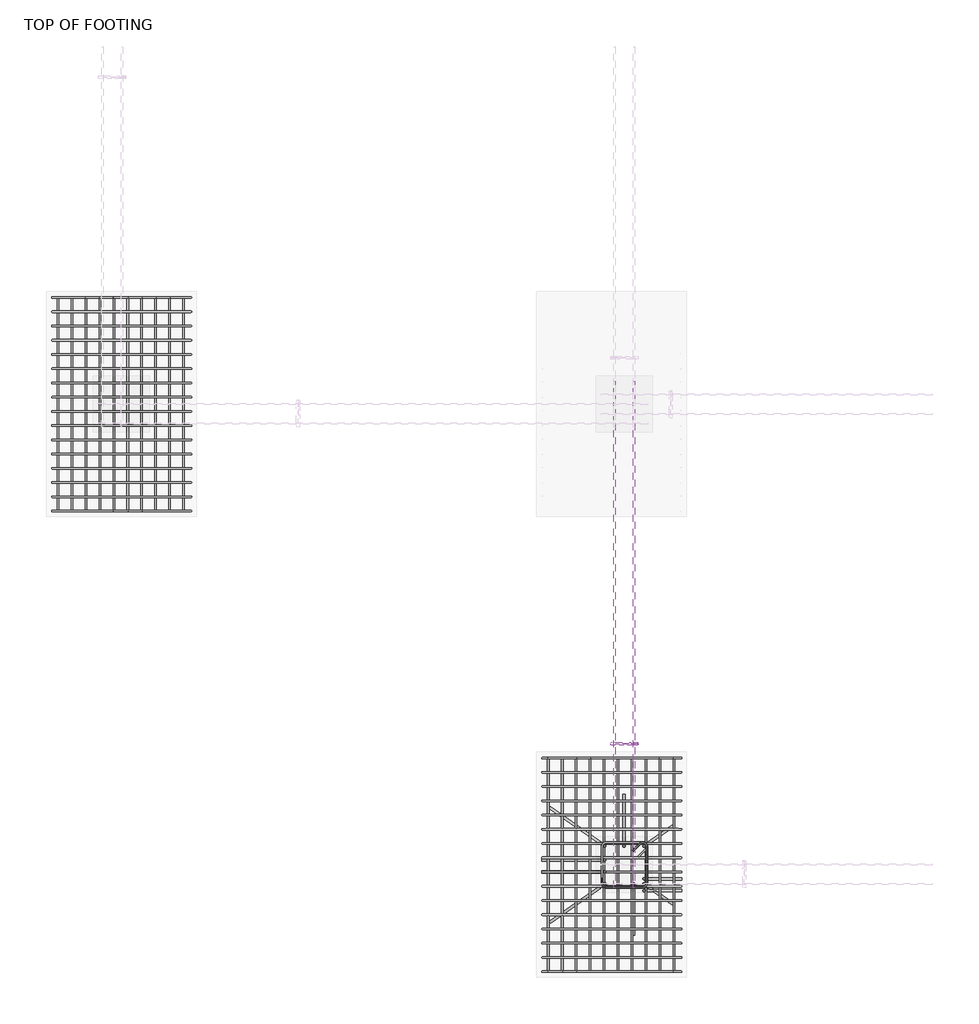
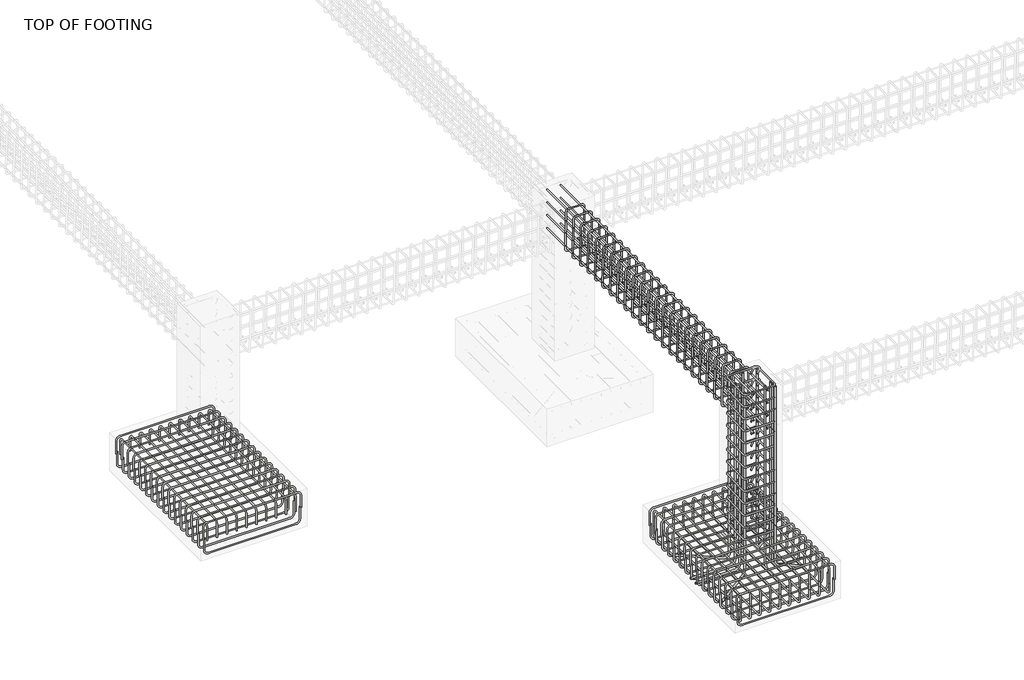
# One storey, part 2 of 11: 19 reinforcing bars.
"""IFC4 building model written with IfcOpenShell, lengths in millimetres."""

from ifc_helpers import new_model, si_unit, point, frame, origin, place, context, project, spatial, polyline, circle_curve, trimmed, segment, composite_curve, source, transform, mapped, element, save
from ifc_brep_helpers import swept_disk

model = new_model("IFC4")

# Units and contexts
model_context = context("Model", 3, world=origin())
ifc_project = project(units=[si_unit("LENGTHUNIT", "METRE", prefix="MILLI")], contexts=[model_context])

# Site, building, storey
site = spatial("IfcSite", under=ifc_project)
building = spatial("IfcBuilding", under=site)
storey = spatial("IfcBuildingStorey", under=building, Name="TOP OF FOOTING", Elevation=-1828.8)

# Reinforcing bars
placement = place(None, origin())
reinforcing_bar_shape = source(origin(), model_context, "Body", "SolidModel", [
    swept_disk(composite_curve([segment(polyline([(-5733.2210247, -2335.4013044, -2046.7466921), (-5733.2210247, -2335.4013044, -2194.0466921)]), True, "CONTINUOUS"), segment(trimmed(circle_curve(frame((-5779.5710247, -2335.4013044, -2194.0466921), z_axis=(0.0, 1.0, 0.0), x_axis=(46.349999999999454, 0.0, 0.0)), 46.35), [point((-5733.2210247, -2335.4013044, -2194.0466921))], [point((-5779.5710247, -2335.4013044, -2240.3966921))], True, "CARTESIAN"), True, "CONTINUOUS"), segment(polyline([(-5779.5710247, -2335.4013044, -2240.3966921), (-6770.7992774, -2335.4013044, -2240.3966921)]), True, "CONTINUOUS"), segment(trimmed(circle_curve(frame((-6770.7992774, -2335.4013044, -2194.0466921), z_axis=(0.0, 1.0, 0.0), x_axis=(0.0, 0.0, -46.34999999999991)), 46.35), [point((-6770.7992774, -2335.4013044, -2240.3966921))], [point((-6817.1492774, -2335.4013044, -2194.0466921))], True, "CARTESIAN"), True, "CONTINUOUS"), segment(polyline([(-6817.1492774, -2335.4013044, -2194.0466921), (-6817.1492774, -2335.4013044, -2046.7466921)]), True, "CONTINUOUS")], self_intersect=False), 6.35),
])
element("IfcReinforcingBar", 1, at=placement, inside=storey, context=model_context, shape_type="MappedRepresentation", body=[
    mapped(reinforcing_bar_shape, transform((0.0, 0.0, 0.0), x_axis=(1.0, 0.0, 0.0), y_axis=(0.0, 1.0, 0.0), z_axis=(0.0, 0.0, 1.0))),
    mapped(reinforcing_bar_shape, transform((0.0, -113.82, 0.0), x_axis=(1.0, 0.0, 0.0), y_axis=(0.0, 1.0, 0.0), z_axis=(0.0, 0.0, 1.0))),
    mapped(reinforcing_bar_shape, transform((0.0, -227.64, 0.0), x_axis=(1.0, 0.0, 0.0), y_axis=(0.0, 1.0, 0.0), z_axis=(0.0, 0.0, 1.0))),
    mapped(reinforcing_bar_shape, transform((0.0, -341.46, 0.0), x_axis=(1.0, 0.0, 0.0), y_axis=(0.0, 1.0, 0.0), z_axis=(0.0, 0.0, 1.0))),
    mapped(reinforcing_bar_shape, transform((0.0, -455.28, 0.0), x_axis=(1.0, 0.0, 0.0), y_axis=(0.0, 1.0, 0.0), z_axis=(0.0, 0.0, 1.0))),
    mapped(reinforcing_bar_shape, transform((0.0, -569.1, 0.0), x_axis=(1.0, 0.0, 0.0), y_axis=(0.0, 1.0, 0.0), z_axis=(0.0, 0.0, 1.0))),
    mapped(reinforcing_bar_shape, transform((0.0, -682.92, 0.0), x_axis=(1.0, 0.0, 0.0), y_axis=(0.0, 1.0, 0.0), z_axis=(0.0, 0.0, 1.0))),
    mapped(reinforcing_bar_shape, transform((0.0, -796.74, 0.0), x_axis=(1.0, 0.0, 0.0), y_axis=(0.0, 1.0, 0.0), z_axis=(0.0, 0.0, 1.0))),
    mapped(reinforcing_bar_shape, transform((0.0, -910.56, 0.0), x_axis=(1.0, 0.0, 0.0), y_axis=(0.0, 1.0, 0.0), z_axis=(0.0, 0.0, 1.0))),
    mapped(reinforcing_bar_shape, transform((0.0, -1024.38, 0.0), x_axis=(1.0, 0.0, 0.0), y_axis=(0.0, 1.0, 0.0), z_axis=(0.0, 0.0, 1.0))),
    mapped(reinforcing_bar_shape, transform((0.0, -1138.2, 0.0), x_axis=(1.0, 0.0, 0.0), y_axis=(0.0, 1.0, 0.0), z_axis=(0.0, 0.0, 1.0))),
    mapped(reinforcing_bar_shape, transform((0.0, -1252.02, 0.0), x_axis=(1.0, 0.0, 0.0), y_axis=(0.0, 1.0, 0.0), z_axis=(0.0, 0.0, 1.0))),
    mapped(reinforcing_bar_shape, transform((0.0, -1365.84, 0.0), x_axis=(1.0, 0.0, 0.0), y_axis=(0.0, 1.0, 0.0), z_axis=(0.0, 0.0, 1.0))),
    mapped(reinforcing_bar_shape, transform((0.0, -1479.66, 0.0), x_axis=(1.0, 0.0, 0.0), y_axis=(0.0, 1.0, 0.0), z_axis=(0.0, 0.0, 1.0))),
    mapped(reinforcing_bar_shape, transform((0.0, -1593.48, 0.0), x_axis=(1.0, 0.0, 0.0), y_axis=(0.0, 1.0, 0.0), z_axis=(0.0, 0.0, 1.0))),
    mapped(reinforcing_bar_shape, transform((0.0, -1707.3, 0.0), x_axis=(1.0, 0.0, 0.0), y_axis=(0.0, 1.0, 0.0), z_axis=(0.0, 0.0, 1.0))),
])
reinforcing_bar_2_shape = source(origin(), model_context, "Body", "SolidModel", [
    swept_disk(composite_curve([segment(polyline([(-6829.0228049, -2335.4013044, -2061.9958198), (-6829.0228049, -2335.4013044, -1914.6958198)]), True, "CONTINUOUS"), segment(trimmed(circle_curve(frame((-6782.6728049, -2335.4013044, -1914.6958198), z_axis=(0.0, 1.0, 0.0), x_axis=(-46.349999999999454, 0.0, 0.0)), 46.35), [point((-6829.0228049, -2335.4013044, -1914.6958198))], [point((-6782.6728049, -2335.4013044, -1868.3458198))], True, "CARTESIAN"), True, "CONTINUOUS"), segment(polyline([(-6782.6728049, -2335.4013044, -1868.3458198), (-5768.0728049, -2335.4013044, -1868.3458198)]), True, "CONTINUOUS"), segment(trimmed(circle_curve(frame((-5768.0728049, -2335.4013044, -1914.6958198), z_axis=(0.0, 1.0, 0.0), x_axis=(0.0, 0.0, 46.34999999999991)), 46.35), [point((-5768.0728049, -2335.4013044, -1868.3458198))], [point((-5721.7228049, -2335.4013044, -1914.6958198))], True, "CARTESIAN"), True, "CONTINUOUS"), segment(polyline([(-5721.7228049, -2335.4013044, -1914.6958198), (-5721.7228049, -2335.4013044, -2061.9958198)]), True, "CONTINUOUS")], self_intersect=False), 6.35),
])
element("IfcReinforcingBar", 2, at=placement, inside=storey, context=model_context, shape_type="MappedRepresentation", body=[
    mapped(reinforcing_bar_2_shape, transform((0.0, 0.0, 0.0), x_axis=(1.0, 0.0, 0.0), y_axis=(0.0, 1.0, 0.0), z_axis=(0.0, 0.0, 1.0))),
    mapped(reinforcing_bar_2_shape, transform((0.0, -113.82, 0.0), x_axis=(1.0, 0.0, 0.0), y_axis=(0.0, 1.0, 0.0), z_axis=(0.0, 0.0, 1.0))),
    mapped(reinforcing_bar_2_shape, transform((0.0, -227.64, 0.0), x_axis=(1.0, 0.0, 0.0), y_axis=(0.0, 1.0, 0.0), z_axis=(0.0, 0.0, 1.0))),
    mapped(reinforcing_bar_2_shape, transform((0.0, -341.46, 0.0), x_axis=(1.0, 0.0, 0.0), y_axis=(0.0, 1.0, 0.0), z_axis=(0.0, 0.0, 1.0))),
    mapped(reinforcing_bar_2_shape, transform((0.0, -455.28, 0.0), x_axis=(1.0, 0.0, 0.0), y_axis=(0.0, 1.0, 0.0), z_axis=(0.0, 0.0, 1.0))),
    mapped(reinforcing_bar_2_shape, transform((0.0, -569.1, 0.0), x_axis=(1.0, 0.0, 0.0), y_axis=(0.0, 1.0, 0.0), z_axis=(0.0, 0.0, 1.0))),
    mapped(reinforcing_bar_2_shape, transform((0.0, -682.92, 0.0), x_axis=(1.0, 0.0, 0.0), y_axis=(0.0, 1.0, 0.0), z_axis=(0.0, 0.0, 1.0))),
    mapped(reinforcing_bar_2_shape, transform((0.0, -796.74, 0.0), x_axis=(1.0, 0.0, 0.0), y_axis=(0.0, 1.0, 0.0), z_axis=(0.0, 0.0, 1.0))),
    mapped(reinforcing_bar_2_shape, transform((0.0, -910.56, 0.0), x_axis=(1.0, 0.0, 0.0), y_axis=(0.0, 1.0, 0.0), z_axis=(0.0, 0.0, 1.0))),
    mapped(reinforcing_bar_2_shape, transform((0.0, -1024.38, 0.0), x_axis=(1.0, 0.0, 0.0), y_axis=(0.0, 1.0, 0.0), z_axis=(0.0, 0.0, 1.0))),
    mapped(reinforcing_bar_2_shape, transform((0.0, -1138.2, 0.0), x_axis=(1.0, 0.0, 0.0), y_axis=(0.0, 1.0, 0.0), z_axis=(0.0, 0.0, 1.0))),
    mapped(reinforcing_bar_2_shape, transform((0.0, -1252.02, 0.0), x_axis=(1.0, 0.0, 0.0), y_axis=(0.0, 1.0, 0.0), z_axis=(0.0, 0.0, 1.0))),
    mapped(reinforcing_bar_2_shape, transform((0.0, -1365.84, 0.0), x_axis=(1.0, 0.0, 0.0), y_axis=(0.0, 1.0, 0.0), z_axis=(0.0, 0.0, 1.0))),
    mapped(reinforcing_bar_2_shape, transform((0.0, -1479.66, 0.0), x_axis=(1.0, 0.0, 0.0), y_axis=(0.0, 1.0, 0.0), z_axis=(0.0, 0.0, 1.0))),
    mapped(reinforcing_bar_2_shape, transform((0.0, -1593.48, 0.0), x_axis=(1.0, 0.0, 0.0), y_axis=(0.0, 1.0, 0.0), z_axis=(0.0, 0.0, 1.0))),
    mapped(reinforcing_bar_2_shape, transform((0.0, -1707.3, 0.0), x_axis=(1.0, 0.0, 0.0), y_axis=(0.0, 1.0, 0.0), z_axis=(0.0, 0.0, 1.0))),
])
reinforcing_bar_3_shape = source(origin(), model_context, "Body", "SolidModel", [
    swept_disk(composite_curve([segment(polyline([(-5779.9394572, -2335.4013044, -2084.0984403), (-5779.9394572, -2335.4013044, -1936.7984403)]), True, "CONTINUOUS"), segment(trimmed(circle_curve(frame((-5779.9394572, -2381.7513044, -1936.7984403), z_axis=(1.0, 0.0, 0.0), x_axis=(0.0, 46.350000000000364, 0.0)), 46.35), [point((-5779.9394572, -2335.4013044, -1936.7984403))], [point((-5779.9394572, -2381.7513044, -1890.4484403))], True, "CARTESIAN"), True, "CONTINUOUS"), segment(polyline([(-5779.9394572, -2381.7513044, -1890.4484403), (-5779.9394572, -3996.3513044, -1890.4484403)]), True, "CONTINUOUS"), segment(trimmed(circle_curve(frame((-5779.9394572, -3996.3513044, -1936.7984403), z_axis=(1.0, 0.0, 0.0), x_axis=(0.0, 0.0, 46.350000000000136)), 46.35), [point((-5779.9394572, -3996.3513044, -1890.4484403))], [point((-5779.9394572, -4042.7013044, -1936.7984403))], True, "CARTESIAN"), True, "CONTINUOUS"), segment(polyline([(-5779.9394572, -4042.7013044, -1936.7984403), (-5779.9394572, -4042.7013044, -2084.0984403)]), True, "CONTINUOUS")], self_intersect=False), 6.35),
])
element("IfcReinforcingBar", 3, at=placement, inside=storey, context=model_context, shape_type="MappedRepresentation", body=[
    mapped(reinforcing_bar_3_shape, transform((0.0, 0.0, 0.0), x_axis=(1.0, 0.0, 0.0), y_axis=(0.0, 1.0, 0.0), z_axis=(0.0, 0.0, 1.0))),
    mapped(reinforcing_bar_3_shape, transform((-111.55177, 0.0, 0.0), x_axis=(1.0, 0.0, 0.0), y_axis=(0.0, 1.0, 0.0), z_axis=(0.0, 0.0, 1.0))),
    mapped(reinforcing_bar_3_shape, transform((-223.10354, 0.0, 0.0), x_axis=(1.0, 0.0, 0.0), y_axis=(0.0, 1.0, 0.0), z_axis=(0.0, 0.0, 1.0))),
    mapped(reinforcing_bar_3_shape, transform((-334.6553099, 0.0, 0.0), x_axis=(1.0, 0.0, 0.0), y_axis=(0.0, 1.0, 0.0), z_axis=(0.0, 0.0, 1.0))),
    mapped(reinforcing_bar_3_shape, transform((-446.2070799, 0.0, 0.0), x_axis=(1.0, 0.0, 0.0), y_axis=(0.0, 1.0, 0.0), z_axis=(0.0, 0.0, 1.0))),
    mapped(reinforcing_bar_3_shape, transform((-557.7588499, 0.0, 0.0), x_axis=(1.0, 0.0, 0.0), y_axis=(0.0, 1.0, 0.0), z_axis=(0.0, 0.0, 1.0))),
    mapped(reinforcing_bar_3_shape, transform((-669.3106199, 0.0, 0.0), x_axis=(1.0, 0.0, 0.0), y_axis=(0.0, 1.0, 0.0), z_axis=(0.0, 0.0, 1.0))),
    mapped(reinforcing_bar_3_shape, transform((-780.8623899, 0.0, 0.0), x_axis=(1.0, 0.0, 0.0), y_axis=(0.0, 1.0, 0.0), z_axis=(0.0, 0.0, 1.0))),
    mapped(reinforcing_bar_3_shape, transform((-892.4141599, 0.0, 0.0), x_axis=(1.0, 0.0, 0.0), y_axis=(0.0, 1.0, 0.0), z_axis=(0.0, 0.0, 1.0))),
    mapped(reinforcing_bar_3_shape, transform((-1003.9659298, 0.0, 0.0), x_axis=(1.0, 0.0, 0.0), y_axis=(0.0, 1.0, 0.0), z_axis=(0.0, 0.0, 1.0))),
])
reinforcing_bar_4_shape = source(origin(), model_context, "Body", "SolidModel", [
    swept_disk(composite_curve([segment(polyline([(-1813.2210247, -6018.1250095, -2046.7466921), (-1813.2210247, -6018.1250095, -2194.0466921)]), True, "CONTINUOUS"), segment(trimmed(circle_curve(frame((-1859.5710247, -6018.1250095, -2194.0466921), z_axis=(0.0, 1.0, 0.0), x_axis=(46.34999999999991, 0.0, 0.0)), 46.35), [point((-1813.2210247, -6018.1250095, -2194.0466921))], [point((-1859.5710247, -6018.1250095, -2240.3966921))], True, "CARTESIAN"), True, "CONTINUOUS"), segment(polyline([(-1859.5710247, -6018.1250095, -2240.3966921), (-2850.7992774, -6018.1250095, -2240.3966921)]), True, "CONTINUOUS"), segment(trimmed(circle_curve(frame((-2850.7992774, -6018.1250095, -2194.0466921), z_axis=(0.0, 1.0, 0.0), x_axis=(0.0, 0.0, -46.34999999999991)), 46.35), [point((-2850.7992774, -6018.1250095, -2240.3966921))], [point((-2897.1492774, -6018.1250095, -2194.0466921))], True, "CARTESIAN"), True, "CONTINUOUS"), segment(polyline([(-2897.1492774, -6018.1250095, -2194.0466921), (-2897.1492774, -6018.1250095, -2046.7466921)]), True, "CONTINUOUS")], self_intersect=False), 6.35),
])
element("IfcReinforcingBar", 4, at=placement, inside=storey, context=model_context, shape_type="MappedRepresentation", body=[
    mapped(reinforcing_bar_4_shape, transform((0.0, 0.0, 0.0), x_axis=(1.0, 0.0, 0.0), y_axis=(0.0, 1.0, 0.0), z_axis=(0.0, 0.0, 1.0))),
    mapped(reinforcing_bar_4_shape, transform((0.0, -113.82, 0.0), x_axis=(1.0, 0.0, 0.0), y_axis=(0.0, 1.0, 0.0), z_axis=(0.0, 0.0, 1.0))),
    mapped(reinforcing_bar_4_shape, transform((0.0, -227.64, 0.0), x_axis=(1.0, 0.0, 0.0), y_axis=(0.0, 1.0, 0.0), z_axis=(0.0, 0.0, 1.0))),
    mapped(reinforcing_bar_4_shape, transform((0.0, -341.46, 0.0), x_axis=(1.0, 0.0, 0.0), y_axis=(0.0, 1.0, 0.0), z_axis=(0.0, 0.0, 1.0))),
    mapped(reinforcing_bar_4_shape, transform((0.0, -455.28, 0.0), x_axis=(1.0, 0.0, 0.0), y_axis=(0.0, 1.0, 0.0), z_axis=(0.0, 0.0, 1.0))),
    mapped(reinforcing_bar_4_shape, transform((0.0, -569.1, 0.0), x_axis=(1.0, 0.0, 0.0), y_axis=(0.0, 1.0, 0.0), z_axis=(0.0, 0.0, 1.0))),
    mapped(reinforcing_bar_4_shape, transform((0.0, -682.92, 0.0), x_axis=(1.0, 0.0, 0.0), y_axis=(0.0, 1.0, 0.0), z_axis=(0.0, 0.0, 1.0))),
    mapped(reinforcing_bar_4_shape, transform((0.0, -796.74, 0.0), x_axis=(1.0, 0.0, 0.0), y_axis=(0.0, 1.0, 0.0), z_axis=(0.0, 0.0, 1.0))),
    mapped(reinforcing_bar_4_shape, transform((0.0, -910.56, 0.0), x_axis=(1.0, 0.0, 0.0), y_axis=(0.0, 1.0, 0.0), z_axis=(0.0, 0.0, 1.0))),
    mapped(reinforcing_bar_4_shape, transform((0.0, -1024.38, 0.0), x_axis=(1.0, 0.0, 0.0), y_axis=(0.0, 1.0, 0.0), z_axis=(0.0, 0.0, 1.0))),
    mapped(reinforcing_bar_4_shape, transform((0.0, -1138.2, 0.0), x_axis=(1.0, 0.0, 0.0), y_axis=(0.0, 1.0, 0.0), z_axis=(0.0, 0.0, 1.0))),
    mapped(reinforcing_bar_4_shape, transform((0.0, -1252.02, 0.0), x_axis=(1.0, 0.0, 0.0), y_axis=(0.0, 1.0, 0.0), z_axis=(0.0, 0.0, 1.0))),
    mapped(reinforcing_bar_4_shape, transform((0.0, -1365.84, 0.0), x_axis=(1.0, 0.0, 0.0), y_axis=(0.0, 1.0, 0.0), z_axis=(0.0, 0.0, 1.0))),
    mapped(reinforcing_bar_4_shape, transform((0.0, -1479.66, 0.0), x_axis=(1.0, 0.0, 0.0), y_axis=(0.0, 1.0, 0.0), z_axis=(0.0, 0.0, 1.0))),
    mapped(reinforcing_bar_4_shape, transform((0.0, -1593.48, 0.0), x_axis=(1.0, 0.0, 0.0), y_axis=(0.0, 1.0, 0.0), z_axis=(0.0, 0.0, 1.0))),
    mapped(reinforcing_bar_4_shape, transform((0.0, -1707.3, 0.0), x_axis=(1.0, 0.0, 0.0), y_axis=(0.0, 1.0, 0.0), z_axis=(0.0, 0.0, 1.0))),
])
reinforcing_bar_5_shape = source(origin(), model_context, "Body", "SolidModel", [
    swept_disk(composite_curve([segment(polyline([(-2909.0228049, -6018.1250095, -2061.9958198), (-2909.0228049, -6018.1250095, -1914.6958198)]), True, "CONTINUOUS"), segment(trimmed(circle_curve(frame((-2862.6728049, -6018.1250095, -1914.6958198), z_axis=(0.0, 1.0, 0.0), x_axis=(-46.350000000000364, 0.0, 0.0)), 46.35), [point((-2909.0228049, -6018.1250095, -1914.6958198))], [point((-2862.6728049, -6018.1250095, -1868.3458198))], True, "CARTESIAN"), True, "CONTINUOUS"), segment(polyline([(-2862.6728049, -6018.1250095, -1868.3458198), (-1848.0728049, -6018.1250095, -1868.3458198)]), True, "CONTINUOUS"), segment(trimmed(circle_curve(frame((-1848.0728049, -6018.1250095, -1914.6958198), z_axis=(0.0, 1.0, 0.0), x_axis=(0.0, 0.0, 46.34999999999991)), 46.35), [point((-1848.0728049, -6018.1250095, -1868.3458198))], [point((-1801.7228049, -6018.1250095, -1914.6958198))], True, "CARTESIAN"), True, "CONTINUOUS"), segment(polyline([(-1801.7228049, -6018.1250095, -1914.6958198), (-1801.7228049, -6018.1250095, -2061.9958198)]), True, "CONTINUOUS")], self_intersect=False), 6.35),
])
element("IfcReinforcingBar", 5, at=placement, inside=storey, context=model_context, shape_type="MappedRepresentation", body=[
    mapped(reinforcing_bar_5_shape, transform((0.0, 0.0, 0.0), x_axis=(1.0, 0.0, 0.0), y_axis=(0.0, 1.0, 0.0), z_axis=(0.0, 0.0, 1.0))),
    mapped(reinforcing_bar_5_shape, transform((0.0, -113.82, 0.0), x_axis=(1.0, 0.0, 0.0), y_axis=(0.0, 1.0, 0.0), z_axis=(0.0, 0.0, 1.0))),
    mapped(reinforcing_bar_5_shape, transform((0.0, -227.64, 0.0), x_axis=(1.0, 0.0, 0.0), y_axis=(0.0, 1.0, 0.0), z_axis=(0.0, 0.0, 1.0))),
    mapped(reinforcing_bar_5_shape, transform((0.0, -341.46, 0.0), x_axis=(1.0, 0.0, 0.0), y_axis=(0.0, 1.0, 0.0), z_axis=(0.0, 0.0, 1.0))),
    mapped(reinforcing_bar_5_shape, transform((0.0, -455.28, 0.0), x_axis=(1.0, 0.0, 0.0), y_axis=(0.0, 1.0, 0.0), z_axis=(0.0, 0.0, 1.0))),
    mapped(reinforcing_bar_5_shape, transform((0.0, -569.1, 0.0), x_axis=(1.0, 0.0, 0.0), y_axis=(0.0, 1.0, 0.0), z_axis=(0.0, 0.0, 1.0))),
    mapped(reinforcing_bar_5_shape, transform((0.0, -682.92, 0.0), x_axis=(1.0, 0.0, 0.0), y_axis=(0.0, 1.0, 0.0), z_axis=(0.0, 0.0, 1.0))),
    mapped(reinforcing_bar_5_shape, transform((0.0, -796.74, 0.0), x_axis=(1.0, 0.0, 0.0), y_axis=(0.0, 1.0, 0.0), z_axis=(0.0, 0.0, 1.0))),
    mapped(reinforcing_bar_5_shape, transform((0.0, -910.56, 0.0), x_axis=(1.0, 0.0, 0.0), y_axis=(0.0, 1.0, 0.0), z_axis=(0.0, 0.0, 1.0))),
    mapped(reinforcing_bar_5_shape, transform((0.0, -1024.38, 0.0), x_axis=(1.0, 0.0, 0.0), y_axis=(0.0, 1.0, 0.0), z_axis=(0.0, 0.0, 1.0))),
    mapped(reinforcing_bar_5_shape, transform((0.0, -1138.2, 0.0), x_axis=(1.0, 0.0, 0.0), y_axis=(0.0, 1.0, 0.0), z_axis=(0.0, 0.0, 1.0))),
    mapped(reinforcing_bar_5_shape, transform((0.0, -1252.02, 0.0), x_axis=(1.0, 0.0, 0.0), y_axis=(0.0, 1.0, 0.0), z_axis=(0.0, 0.0, 1.0))),
    mapped(reinforcing_bar_5_shape, transform((0.0, -1365.84, 0.0), x_axis=(1.0, 0.0, 0.0), y_axis=(0.0, 1.0, 0.0), z_axis=(0.0, 0.0, 1.0))),
    mapped(reinforcing_bar_5_shape, transform((0.0, -1479.66, 0.0), x_axis=(1.0, 0.0, 0.0), y_axis=(0.0, 1.0, 0.0), z_axis=(0.0, 0.0, 1.0))),
    mapped(reinforcing_bar_5_shape, transform((0.0, -1593.48, 0.0), x_axis=(1.0, 0.0, 0.0), y_axis=(0.0, 1.0, 0.0), z_axis=(0.0, 0.0, 1.0))),
    mapped(reinforcing_bar_5_shape, transform((0.0, -1707.3, 0.0), x_axis=(1.0, 0.0, 0.0), y_axis=(0.0, 1.0, 0.0), z_axis=(0.0, 0.0, 1.0))),
])
reinforcing_bar_6_shape = source(origin(), model_context, "Body", "SolidModel", [
    swept_disk(composite_curve([segment(polyline([(-1859.9394572, -6018.1250095, -2084.0984403), (-1859.9394572, -6018.1250095, -1936.7984403)]), True, "CONTINUOUS"), segment(trimmed(circle_curve(frame((-1859.9394572, -6064.4750095, -1936.7984403), z_axis=(1.0, 0.0, 0.0), x_axis=(0.0, 46.350000000000364, 0.0)), 46.35), [point((-1859.9394572, -6018.1250095, -1936.7984403))], [point((-1859.9394572, -6064.4750095, -1890.4484403))], True, "CARTESIAN"), True, "CONTINUOUS"), segment(polyline([(-1859.9394572, -6064.4750095, -1890.4484403), (-1859.9394572, -7679.0750095, -1890.4484403)]), True, "CONTINUOUS"), segment(trimmed(circle_curve(frame((-1859.9394572, -7679.0750095, -1936.7984403), z_axis=(1.0, 0.0, 0.0), x_axis=(0.0, 0.0, 46.350000000000136)), 46.35), [point((-1859.9394572, -7679.0750095, -1890.4484403))], [point((-1859.9394572, -7725.4250095, -1936.7984403))], True, "CARTESIAN"), True, "CONTINUOUS"), segment(polyline([(-1859.9394572, -7725.4250095, -1936.7984403), (-1859.9394572, -7725.4250095, -2084.0984403)]), True, "CONTINUOUS")], self_intersect=False), 6.35),
])
element("IfcReinforcingBar", 6, at=placement, inside=storey, context=model_context, shape_type="MappedRepresentation", body=[
    mapped(reinforcing_bar_6_shape, transform((0.0, 0.0, 0.0), x_axis=(1.0, 0.0, 0.0), y_axis=(0.0, 1.0, 0.0), z_axis=(0.0, 0.0, 1.0))),
    mapped(reinforcing_bar_6_shape, transform((-111.55177, 0.0, 0.0), x_axis=(1.0, 0.0, 0.0), y_axis=(0.0, 1.0, 0.0), z_axis=(0.0, 0.0, 1.0))),
    mapped(reinforcing_bar_6_shape, transform((-223.10354, 0.0, 0.0), x_axis=(1.0, 0.0, 0.0), y_axis=(0.0, 1.0, 0.0), z_axis=(0.0, 0.0, 1.0))),
    mapped(reinforcing_bar_6_shape, transform((-334.6553099, 0.0, 0.0), x_axis=(1.0, 0.0, 0.0), y_axis=(0.0, 1.0, 0.0), z_axis=(0.0, 0.0, 1.0))),
    mapped(reinforcing_bar_6_shape, transform((-446.2070799, 0.0, 0.0), x_axis=(1.0, 0.0, 0.0), y_axis=(0.0, 1.0, 0.0), z_axis=(0.0, 0.0, 1.0))),
    mapped(reinforcing_bar_6_shape, transform((-557.7588499, 0.0, 0.0), x_axis=(1.0, 0.0, 0.0), y_axis=(0.0, 1.0, 0.0), z_axis=(0.0, 0.0, 1.0))),
    mapped(reinforcing_bar_6_shape, transform((-669.3106199, 0.0, 0.0), x_axis=(1.0, 0.0, 0.0), y_axis=(0.0, 1.0, 0.0), z_axis=(0.0, 0.0, 1.0))),
    mapped(reinforcing_bar_6_shape, transform((-780.8623899, 0.0, 0.0), x_axis=(1.0, 0.0, 0.0), y_axis=(0.0, 1.0, 0.0), z_axis=(0.0, 0.0, 1.0))),
    mapped(reinforcing_bar_6_shape, transform((-892.4141599, 0.0, 0.0), x_axis=(1.0, 0.0, 0.0), y_axis=(0.0, 1.0, 0.0), z_axis=(0.0, 0.0, 1.0))),
    mapped(reinforcing_bar_6_shape, transform((-1003.9659298, 0.0, 0.0), x_axis=(1.0, 0.0, 0.0), y_axis=(0.0, 1.0, 0.0), z_axis=(0.0, 0.0, 1.0))),
])
reinforcing_bar_7_shape = source(origin(), model_context, "Body", "SolidModel", [
    swept_disk(composite_curve([segment(polyline([(-2863.9053871, -6018.1250095, -2021.5298587), (-2863.9053871, -6018.1250095, -2168.8298587)]), True, "CONTINUOUS"), segment(trimmed(circle_curve(frame((-2863.9053871, -6064.4750095, -2168.8298587), z_axis=(-1.0, 0.0, 0.0), x_axis=(0.0, 46.350000000000364, 0.0)), 46.35), [point((-2863.9053871, -6018.1250095, -2168.8298587))], [point((-2863.9053871, -6064.4750095, -2215.1798587))], True, "CARTESIAN"), True, "CONTINUOUS"), segment(polyline([(-2863.9053871, -6064.4750095, -2215.1798587), (-2863.9053871, -7679.0750095, -2215.1798587)]), True, "CONTINUOUS"), segment(trimmed(circle_curve(frame((-2863.9053871, -7679.0750095, -2168.8298587), z_axis=(-1.0, 0.0, 0.0), x_axis=(0.0, 0.0, -46.34999999999991)), 46.35), [point((-2863.9053871, -7679.0750095, -2215.1798587))], [point((-2863.9053871, -7725.4250095, -2168.8298587))], True, "CARTESIAN"), True, "CONTINUOUS"), segment(polyline([(-2863.9053871, -7725.4250095, -2168.8298587), (-2863.9053871, -7725.4250095, -2021.5298587)]), True, "CONTINUOUS")], self_intersect=False), 6.35),
])
element("IfcReinforcingBar", 7, at=placement, inside=storey, context=model_context, shape_type="MappedRepresentation", body=[
    mapped(reinforcing_bar_7_shape, transform((0.0, 0.0, 0.0), x_axis=(1.0, 0.0, 0.0), y_axis=(0.0, 1.0, 0.0), z_axis=(0.0, 0.0, 1.0))),
    mapped(reinforcing_bar_7_shape, transform((111.55177, 0.0, 0.0), x_axis=(1.0, 0.0, 0.0), y_axis=(0.0, 1.0, 0.0), z_axis=(0.0, 0.0, 1.0))),
    mapped(reinforcing_bar_7_shape, transform((223.10354, 0.0, 0.0), x_axis=(1.0, 0.0, 0.0), y_axis=(0.0, 1.0, 0.0), z_axis=(0.0, 0.0, 1.0))),
    mapped(reinforcing_bar_7_shape, transform((334.6553099, 0.0, 0.0), x_axis=(1.0, 0.0, 0.0), y_axis=(0.0, 1.0, 0.0), z_axis=(0.0, 0.0, 1.0))),
    mapped(reinforcing_bar_7_shape, transform((446.2070799, 0.0, 0.0), x_axis=(1.0, 0.0, 0.0), y_axis=(0.0, 1.0, 0.0), z_axis=(0.0, 0.0, 1.0))),
    mapped(reinforcing_bar_7_shape, transform((557.7588499, 0.0, 0.0), x_axis=(1.0, 0.0, 0.0), y_axis=(0.0, 1.0, 0.0), z_axis=(0.0, 0.0, 1.0))),
    mapped(reinforcing_bar_7_shape, transform((669.3106199, 0.0, 0.0), x_axis=(1.0, 0.0, 0.0), y_axis=(0.0, 1.0, 0.0), z_axis=(0.0, 0.0, 1.0))),
    mapped(reinforcing_bar_7_shape, transform((780.8623899, 0.0, 0.0), x_axis=(1.0, 0.0, 0.0), y_axis=(0.0, 1.0, 0.0), z_axis=(0.0, 0.0, 1.0))),
    mapped(reinforcing_bar_7_shape, transform((892.4141599, 0.0, 0.0), x_axis=(1.0, 0.0, 0.0), y_axis=(0.0, 1.0, 0.0), z_axis=(0.0, 0.0, 1.0))),
    mapped(reinforcing_bar_7_shape, transform((1003.9659298, 0.0, 0.0), x_axis=(1.0, 0.0, 0.0), y_axis=(0.0, 1.0, 0.0), z_axis=(0.0, 0.0, 1.0))),
])
reinforcing_bar_8_shape = source(origin(), model_context, "Body", "SolidModel", [
    swept_disk(composite_curve([segment(polyline([(-2185.9841654, -6758.0507749, -46.35), (-2130.2406025, -6702.3072119, -46.35)]), True, "CONTINUOUS"), segment(trimmed(circle_curve(frame((-2108.0728049, -6724.4750095, -46.35), z_axis=(0.0, 0.0, -1.0), x_axis=(-22.167797600000085, 22.167797600000085, 0.0)), 31.35), [point((-2130.2406025, -6702.3072119, -46.35))], [point((-2076.7228049, -6724.4750095, -46.35))], True, "CARTESIAN"), True, "CONTINUOUS"), segment(polyline([(-2076.7228049, -6724.4750095, -46.35), (-2076.7228049, -7019.0750095, -46.35)]), True, "CONTINUOUS"), segment(trimmed(circle_curve(frame((-2108.0728049, -7019.0750095, -46.35), z_axis=(0.0, 0.0, -1.0), x_axis=(31.34999999999991, 0.0, 0.0)), 31.35), [point((-2076.7228049, -7019.0750095, -46.35))], [point((-2108.0728049, -7050.4250095, -46.35))], True, "CARTESIAN"), True, "CONTINUOUS"), segment(polyline([(-2108.0728049, -7050.4250095, -46.35), (-2402.6728049, -7050.4250095, -46.35)]), True, "CONTINUOUS"), segment(trimmed(circle_curve(frame((-2402.6728049, -7019.0947946, -45.2363875), z_axis=(0.0, 0.03552192833448201, -0.9993688971583016), x_axis=(0.0, -31.3302149000001, -1.1136125000000021)), 31.35), [point((-2402.6728049, -7050.4250095, -46.35))], [point((-2434.0228049, -7019.0947946, -45.2363875))], True, "CARTESIAN"), True, "CONTINUOUS"), segment(polyline([(-2434.0228049, -7019.0947946, -45.2363875), (-2434.0228049, -6724.4552244, -34.7636125)]), True, "CONTINUOUS"), segment(trimmed(circle_curve(frame((-2402.6728049, -6724.4552244, -34.7636125), z_axis=(0.0, 0.03552192833448201, -0.9993688971583016), x_axis=(-31.350000000000364, 0.0, 0.0)), 31.35), [point((-2434.0228049, -6724.4552244, -34.7636125))], [point((-2402.6728049, -6693.1250095, -33.65))], True, "CARTESIAN"), True, "CONTINUOUS"), segment(polyline([(-2402.6728049, -6693.1250095, -33.65), (-2108.0728049, -6693.1250095, -33.65)]), True, "CONTINUOUS"), segment(trimmed(circle_curve(frame((-2108.0728049, -6724.4750095, -33.65), z_axis=(0.0, 0.0, -1.0), x_axis=(0.0, 31.350000000000364, 0.0)), 31.35), [point((-2108.0728049, -6693.1250095, -33.65))], [point((-2085.9050073, -6746.6428071, -33.65))], True, "CARTESIAN"), True, "CONTINUOUS"), segment(polyline([(-2085.9050073, -6746.6428071, -33.65), (-2141.6485703, -6802.3863701, -33.65)]), True, "CONTINUOUS")], self_intersect=False), 6.35),
])
element("IfcReinforcingBar", 8, at=placement, inside=storey, context=model_context, shape_type="MappedRepresentation", body=[
    mapped(reinforcing_bar_8_shape, transform((0.0, 0.0, 0.0), x_axis=(1.0, 0.0, 0.0), y_axis=(0.0, 1.0, 0.0), z_axis=(0.0, 0.0, 1.0))),
    mapped(reinforcing_bar_8_shape, transform((0.0, 0.0, -144.675), x_axis=(1.0, 0.0, 0.0), y_axis=(0.0, 1.0, 0.0), z_axis=(0.0, 0.0, 1.0))),
    mapped(reinforcing_bar_8_shape, transform((0.0, 0.0, -289.35), x_axis=(1.0, 0.0, 0.0), y_axis=(0.0, 1.0, 0.0), z_axis=(0.0, 0.0, 1.0))),
    mapped(reinforcing_bar_8_shape, transform((0.0, 0.0, -434.025), x_axis=(1.0, 0.0, 0.0), y_axis=(0.0, 1.0, 0.0), z_axis=(0.0, 0.0, 1.0))),
    mapped(reinforcing_bar_8_shape, transform((0.0, 0.0, -578.7), x_axis=(1.0, 0.0, 0.0), y_axis=(0.0, 1.0, 0.0), z_axis=(0.0, 0.0, 1.0))),
    mapped(reinforcing_bar_8_shape, transform((0.0, 0.0, -723.375), x_axis=(1.0, 0.0, 0.0), y_axis=(0.0, 1.0, 0.0), z_axis=(0.0, 0.0, 1.0))),
    mapped(reinforcing_bar_8_shape, transform((0.0, 0.0, -868.05), x_axis=(1.0, 0.0, 0.0), y_axis=(0.0, 1.0, 0.0), z_axis=(0.0, 0.0, 1.0))),
    mapped(reinforcing_bar_8_shape, transform((0.0, 0.0, -1012.725), x_axis=(1.0, 0.0, 0.0), y_axis=(0.0, 1.0, 0.0), z_axis=(0.0, 0.0, 1.0))),
    mapped(reinforcing_bar_8_shape, transform((0.0, 0.0, -1157.4), x_axis=(1.0, 0.0, 0.0), y_axis=(0.0, 1.0, 0.0), z_axis=(0.0, 0.0, 1.0))),
    mapped(reinforcing_bar_8_shape, transform((0.0, 0.0, -1302.075), x_axis=(1.0, 0.0, 0.0), y_axis=(0.0, 1.0, 0.0), z_axis=(0.0, 0.0, 1.0))),
    mapped(reinforcing_bar_8_shape, transform((0.0, 0.0, -1446.75), x_axis=(1.0, 0.0, 0.0), y_axis=(0.0, 1.0, 0.0), z_axis=(0.0, 0.0, 1.0))),
    mapped(reinforcing_bar_8_shape, transform((0.0, 0.0, -1591.425), x_axis=(1.0, 0.0, 0.0), y_axis=(0.0, 1.0, 0.0), z_axis=(0.0, 0.0, 1.0))),
    mapped(reinforcing_bar_8_shape, transform((0.0, 0.0, -1736.1), x_axis=(1.0, 0.0, 0.0), y_axis=(0.0, 1.0, 0.0), z_axis=(0.0, 0.0, 1.0))),
])
reinforcing_bar_9_shape = source(origin(), model_context, "Body", "SolidModel", [
    swept_disk(composite_curve([segment(polyline([(-2098.0728049, -6983.1823983, -40.0), (-2098.0728049, -6983.1823983, -2136.75)]), True, "CONTINUOUS"), segment(trimmed(circle_curve(frame((-2031.0228049, -6983.1823983, -2136.75), z_axis=(0.0, -1.0, 0.0), x_axis=(-67.04999999999995, 0.0, 0.0)), 67.05), [point((-2098.0728049, -6983.1823983, -2136.75))], [point((-2031.0228049, -6983.1823983, -2203.8))], True, "CARTESIAN"), True, "CONTINUOUS"), segment(polyline([(-2031.0228049, -6983.1823983, -2203.8), (-1795.3728049, -6983.1823983, -2203.8)]), True, "CONTINUOUS")], self_intersect=False), 9.55),
])
element("IfcReinforcingBar", 9, at=placement, inside=storey, context=model_context, shape_type="MappedRepresentation", body=[
    mapped(reinforcing_bar_9_shape, transform((0.0, 0.0, 0.0), x_axis=(1.0, 0.0, 0.0), y_axis=(0.0, 1.0, 0.0), z_axis=(0.0, 0.0, 1.0))),
    mapped(reinforcing_bar_9_shape, transform((0.0, -94.3634327, 0.0), x_axis=(1.0, 0.0, 0.0), y_axis=(0.0, 1.0, 0.0), z_axis=(0.0, 0.0, 1.0))),
])
element("IfcReinforcingBar", 10, at=placement, inside=storey, context=model_context, shape_type="SolidModel", body=[
    swept_disk(composite_curve([segment(polyline([(-2098.0728049, -7022.7250095, -40.0), (-2098.0728049, -7022.7250095, -2136.75)]), True, "CONTINUOUS"), segment(trimmed(circle_curve(frame((-2043.1486603, -7061.1833096, -2136.75), z_axis=(-0.5735764363510477, -0.8191520442889908, 0.0), x_axis=(-54.92414459999986, 38.45830010000009, 0.0)), 67.05), [point((-2098.0728049, -7022.7250095, -2136.75))], [point((-2043.1486603, -7061.1833096, -2203.8))], True, "CARTESIAN"), True, "CONTINUOUS"), segment(polyline([(-2043.1486603, -7061.1833096, -2203.8), (-1860.0087562, -7189.419251, -2203.8)]), True, "CONTINUOUS")], self_intersect=False), 9.55),
])
element("IfcReinforcingBar", 11, at=placement, inside=storey, context=model_context, shape_type="SolidModel", body=[
    swept_disk(composite_curve([segment(polyline([(-2098.0728049, -6720.8250095, -40.0), (-2098.0728049, -6720.8250095, -2136.75)]), True, "CONTINUOUS"), segment(trimmed(circle_curve(frame((-2043.1486603, -6682.3667095, -2136.75), z_axis=(0.5735764363510477, -0.8191520442889908, 0.0), x_axis=(-54.92414459999986, -38.458300000000236, 0.0)), 67.05), [point((-2098.0728049, -6720.8250095, -2136.75))], [point((-2043.1486603, -6682.3667095, -2203.8))], True, "CARTESIAN"), True, "CONTINUOUS"), segment(polyline([(-2043.1486603, -6682.3667095, -2203.8), (-1860.0087562, -6554.1307681, -2203.8)]), True, "CONTINUOUS")], self_intersect=False), 9.55),
])
element("IfcReinforcingBar", 12, at=placement, inside=storey, context=model_context, shape_type="SolidModel", body=[
    swept_disk(composite_curve([segment(polyline([(-2412.6728049, -7022.7250095, -40.0), (-2412.6728049, -7022.7250095, -2136.75)]), True, "CONTINUOUS"), segment(trimmed(circle_curve(frame((-2467.5969495, -7061.1833096, -2136.75), z_axis=(-0.5735764363510477, 0.8191520442889908, 0.0), x_axis=(54.92414460000009, 38.45830010000009, 0.0)), 67.05), [point((-2412.6728049, -7022.7250095, -2136.75))], [point((-2467.5969495, -7061.1833096, -2203.8))], True, "CARTESIAN"), True, "CONTINUOUS"), segment(polyline([(-2467.5969495, -7061.1833096, -2203.8), (-2850.7368536, -7329.4607586, -2203.8)]), True, "CONTINUOUS")], self_intersect=False), 9.55),
])
element("IfcReinforcingBar", 13, at=placement, inside=storey, context=model_context, shape_type="SolidModel", body=[
    swept_disk(composite_curve([segment(polyline([(-2412.6728049, -6720.8250095, -40.0), (-2412.6728049, -6720.8250095, -2136.75)]), True, "CONTINUOUS"), segment(trimmed(circle_curve(frame((-2467.5969495, -6682.3667095, -2136.75), z_axis=(0.5735764363510477, 0.8191520442889907, 0.0), x_axis=(54.92414460000009, -38.458300000000236, 0.0)), 67.05), [point((-2412.6728049, -6720.8250095, -2136.75))], [point((-2467.5969495, -6682.3667095, -2203.8))], True, "CARTESIAN"), True, "CONTINUOUS"), segment(polyline([(-2467.5969495, -6682.3667095, -2203.8), (-2850.7368536, -6414.0892604, -2203.8)]), True, "CONTINUOUS")], self_intersect=False), 9.55),
])
reinforcing_bar_10_shape = source(origin(), model_context, "Body", "SolidModel", [
    swept_disk(composite_curve([segment(polyline([(-2412.6728049, -6833.1823983, -40.0), (-2412.6728049, -6833.1823983, -2136.75)]), True, "CONTINUOUS"), segment(trimmed(circle_curve(frame((-2479.7228049, -6833.1823983, -2136.75), z_axis=(0.0, 1.0, 0.0), x_axis=(67.05000000000018, 0.0, 0.0)), 67.05), [point((-2412.6728049, -6833.1823983, -2136.75))], [point((-2479.7228049, -6833.1823983, -2203.8))], True, "CARTESIAN"), True, "CONTINUOUS"), segment(polyline([(-2479.7228049, -6833.1823983, -2203.8), (-2915.3728049, -6833.1823983, -2203.8)]), True, "CONTINUOUS")], self_intersect=False), 9.55),
])
element("IfcReinforcingBar", 14, at=placement, inside=storey, context=model_context, shape_type="MappedRepresentation", body=[
    mapped(reinforcing_bar_10_shape, transform((0.0, 0.0, 0.0), x_axis=(1.0, 0.0, 0.0), y_axis=(0.0, 1.0, 0.0), z_axis=(0.0, 0.0, 1.0))),
    mapped(reinforcing_bar_10_shape, transform((0.0, -94.3634327, 0.0), x_axis=(1.0, 0.0, 0.0), y_axis=(0.0, 1.0, 0.0), z_axis=(0.0, 0.0, 1.0))),
])
element("IfcReinforcingBar", 15, at=placement, inside=storey, context=model_context, shape_type="SolidModel", body=[
    swept_disk(composite_curve([segment(polyline([(-2258.0728049, -6720.8250095, -40.0), (-2258.0728049, -6720.8250095, -2136.75)]), True, "CONTINUOUS"), segment(trimmed(circle_curve(frame((-2258.0728049, -6653.7750095, -2136.75), z_axis=(1.0, 0.0, 0.0), x_axis=(0.0, -67.05000000000018, 0.0)), 67.05), [point((-2258.0728049, -6720.8250095, -2136.75))], [point((-2258.0728049, -6653.7750095, -2203.8))], True, "CARTESIAN"), True, "CONTINUOUS"), segment(polyline([(-2258.0728049, -6653.7750095, -2203.8), (-2258.0728049, -6308.1250095, -2203.8)]), True, "CONTINUOUS")], self_intersect=False), 9.55),
])
element("IfcReinforcingBar", 16, at=placement, inside=storey, context=model_context, shape_type="SolidModel", body=[
    swept_disk(composite_curve([segment(polyline([(-2183.0728049, -7022.7250095, -40.0), (-2183.0728049, -7022.7250095, -2136.75)]), True, "CONTINUOUS"), segment(trimmed(circle_curve(frame((-2183.0728049, -7089.7750095, -2136.75), z_axis=(-1.0, 0.0, 0.0), x_axis=(0.0, 67.05000000000018, 0.0)), 67.05), [point((-2183.0728049, -7022.7250095, -2136.75))], [point((-2183.0728049, -7089.7750095, -2203.8))], True, "CARTESIAN"), True, "CONTINUOUS"), segment(polyline([(-2183.0728049, -7089.7750095, -2203.8), (-2183.0728049, -7435.4250095, -2203.8)]), True, "CONTINUOUS")], self_intersect=False), 9.55),
])
reinforcing_bar_11_shape = source(origin(), model_context, "Body", "SolidModel", [
    swept_disk(composite_curve([segment(polyline([(-2260.9841654, -3420.4013044, -488.7242346), (-2205.2406025, -3420.4013044, -544.4677976)]), True, "CONTINUOUS"), segment(trimmed(circle_curve(frame((-2183.0728049, -3420.4013044, -522.3), z_axis=(0.0, -1.0, 0.0), x_axis=(-22.167797600000085, 0.0, -22.167797600000085)), 31.35), [point((-2205.2406025, -3420.4013044, -544.4677976))], [point((-2151.7228049, -3420.4013044, -522.3))], True, "CARTESIAN"), True, "CONTINUOUS"), segment(polyline([(-2151.7228049, -3420.4013044, -522.3), (-2151.7228049, -3420.4013044, -77.7)]), True, "CONTINUOUS"), segment(trimmed(circle_curve(frame((-2183.0728049, -3420.4013044, -77.7), z_axis=(0.0, -1.0, 0.0), x_axis=(31.34999999999991, 0.0, 0.0)), 31.35), [point((-2151.7228049, -3420.4013044, -77.7))], [point((-2183.0728049, -3420.4013044, -46.35))], True, "CARTESIAN"), True, "CONTINUOUS"), segment(polyline([(-2183.0728049, -3420.4013044, -46.35), (-2327.6728049, -3420.4013044, -46.35)]), True, "CONTINUOUS"), segment(trimmed(circle_curve(frame((-2327.6728049, -3419.6167188, -77.6901807), z_axis=(0.0, -0.9996867842138424, -0.025026655153786322), x_axis=(0.0, -0.7845855999999003, 31.340180699999998)), 31.35), [point((-2327.6728049, -3420.4013044, -46.35))], [point((-2359.0228049, -3419.6167188, -77.6901807))], True, "CARTESIAN"), True, "CONTINUOUS"), segment(polyline([(-2359.0228049, -3419.6167188, -77.6901807), (-2359.0228049, -3408.48589, -522.3098193)]), True, "CONTINUOUS"), segment(trimmed(circle_curve(frame((-2327.6728049, -3408.48589, -522.3098193), z_axis=(0.0, -0.9996867842138424, -0.025026655153786322), x_axis=(-31.350000000000364, 0.0, 0.0)), 31.35), [point((-2359.0228049, -3408.48589, -522.3098193))], [point((-2327.6728049, -3407.7013044, -553.65))], True, "CARTESIAN"), True, "CONTINUOUS"), segment(polyline([(-2327.6728049, -3407.7013044, -553.65), (-2183.0728049, -3407.7013044, -553.65)]), True, "CONTINUOUS"), segment(trimmed(circle_curve(frame((-2183.0728049, -3407.7013044, -522.3), z_axis=(0.0, -1.0, 0.0), x_axis=(0.0, 0.0, -31.350000000000023)), 31.35), [point((-2183.0728049, -3407.7013044, -553.65))], [point((-2160.9050073, -3407.7013044, -500.1322024))], True, "CARTESIAN"), True, "CONTINUOUS"), segment(polyline([(-2160.9050073, -3407.7013044, -500.1322024), (-2216.6485703, -3407.7013044, -444.3886395)]), True, "CONTINUOUS")], self_intersect=False), 6.35),
])
element("IfcReinforcingBar", 17, at=placement, inside=storey, context=model_context, shape_type="MappedRepresentation", body=[
    mapped(reinforcing_bar_11_shape, transform((0.0, 0.0, 0.0), x_axis=(1.0, 0.0, 0.0), y_axis=(0.0, 1.0, 0.0), z_axis=(0.0, 0.0, 1.0))),
    mapped(reinforcing_bar_11_shape, transform((0.0, -146.3647139, 0.0), x_axis=(1.0, 0.0, 0.0), y_axis=(0.0, 1.0, 0.0), z_axis=(0.0, 0.0, 1.0))),
    mapped(reinforcing_bar_11_shape, transform((0.0, -292.7294277, 0.0), x_axis=(1.0, 0.0, 0.0), y_axis=(0.0, 1.0, 0.0), z_axis=(0.0, 0.0, 1.0))),
    mapped(reinforcing_bar_11_shape, transform((0.0, -439.0941416, 0.0), x_axis=(1.0, 0.0, 0.0), y_axis=(0.0, 1.0, 0.0), z_axis=(0.0, 0.0, 1.0))),
    mapped(reinforcing_bar_11_shape, transform((0.0, -585.4588555, 0.0), x_axis=(1.0, 0.0, 0.0), y_axis=(0.0, 1.0, 0.0), z_axis=(0.0, 0.0, 1.0))),
    mapped(reinforcing_bar_11_shape, transform((0.0, -731.8235693, 0.0), x_axis=(1.0, 0.0, 0.0), y_axis=(0.0, 1.0, 0.0), z_axis=(0.0, 0.0, 1.0))),
    mapped(reinforcing_bar_11_shape, transform((0.0, -878.1882832, 0.0), x_axis=(1.0, 0.0, 0.0), y_axis=(0.0, 1.0, 0.0), z_axis=(0.0, 0.0, 1.0))),
    mapped(reinforcing_bar_11_shape, transform((0.0, -1024.5529971, 0.0), x_axis=(1.0, 0.0, 0.0), y_axis=(0.0, 1.0, 0.0), z_axis=(0.0, 0.0, 1.0))),
    mapped(reinforcing_bar_11_shape, transform((0.0, -1170.917711, 0.0), x_axis=(1.0, 0.0, 0.0), y_axis=(0.0, 1.0, 0.0), z_axis=(0.0, 0.0, 1.0))),
    mapped(reinforcing_bar_11_shape, transform((0.0, -1317.2824248, 0.0), x_axis=(1.0, 0.0, 0.0), y_axis=(0.0, 1.0, 0.0), z_axis=(0.0, 0.0, 1.0))),
    mapped(reinforcing_bar_11_shape, transform((0.0, -1463.6471387, 0.0), x_axis=(1.0, 0.0, 0.0), y_axis=(0.0, 1.0, 0.0), z_axis=(0.0, 0.0, 1.0))),
    mapped(reinforcing_bar_11_shape, transform((0.0, -1610.0118526, 0.0), x_axis=(1.0, 0.0, 0.0), y_axis=(0.0, 1.0, 0.0), z_axis=(0.0, 0.0, 1.0))),
    mapped(reinforcing_bar_11_shape, transform((0.0, -1756.3765664, 0.0), x_axis=(1.0, 0.0, 0.0), y_axis=(0.0, 1.0, 0.0), z_axis=(0.0, 0.0, 1.0))),
    mapped(reinforcing_bar_11_shape, transform((0.0, -1902.7412803, 0.0), x_axis=(1.0, 0.0, 0.0), y_axis=(0.0, 1.0, 0.0), z_axis=(0.0, 0.0, 1.0))),
    mapped(reinforcing_bar_11_shape, transform((0.0, -2049.1059942, 0.0), x_axis=(1.0, 0.0, 0.0), y_axis=(0.0, 1.0, 0.0), z_axis=(0.0, 0.0, 1.0))),
    mapped(reinforcing_bar_11_shape, transform((0.0, -2195.470708, 0.0), x_axis=(1.0, 0.0, 0.0), y_axis=(0.0, 1.0, 0.0), z_axis=(0.0, 0.0, 1.0))),
    mapped(reinforcing_bar_11_shape, transform((0.0, -2341.8354219, 0.0), x_axis=(1.0, 0.0, 0.0), y_axis=(0.0, 1.0, 0.0), z_axis=(0.0, 0.0, 1.0))),
    mapped(reinforcing_bar_11_shape, transform((0.0, -2488.2001358, 0.0), x_axis=(1.0, 0.0, 0.0), y_axis=(0.0, 1.0, 0.0), z_axis=(0.0, 0.0, 1.0))),
    mapped(reinforcing_bar_11_shape, transform((0.0, -2634.5648497, 0.0), x_axis=(1.0, 0.0, 0.0), y_axis=(0.0, 1.0, 0.0), z_axis=(0.0, 0.0, 1.0))),
    mapped(reinforcing_bar_11_shape, transform((0.0, -2780.9295635, 0.0), x_axis=(1.0, 0.0, 0.0), y_axis=(0.0, 1.0, 0.0), z_axis=(0.0, 0.0, 1.0))),
    mapped(reinforcing_bar_11_shape, transform((0.0, -2927.2942774, 0.0), x_axis=(1.0, 0.0, 0.0), y_axis=(0.0, 1.0, 0.0), z_axis=(0.0, 0.0, 1.0))),
    mapped(reinforcing_bar_11_shape, transform((0.0, -3073.6589913, 0.0), x_axis=(1.0, 0.0, 0.0), y_axis=(0.0, 1.0, 0.0), z_axis=(0.0, 0.0, 1.0))),
    mapped(reinforcing_bar_11_shape, transform((0.0, -3220.0237051, 0.0), x_axis=(1.0, 0.0, 0.0), y_axis=(0.0, 1.0, 0.0), z_axis=(0.0, 0.0, 1.0))),
])
reinforcing_bar_12_shape = source(origin(), model_context, "Body", "SolidModel", [
    swept_disk(composite_curve([segment(polyline([(-2178.0728049, -3004.0513044, -528.2977114), (-2178.0728049, -7056.7750095, -528.2977114)]), True, "CONTINUOUS")], self_intersect=False), 6.35),
])
element("IfcReinforcingBar", 18, at=placement, inside=storey, context=model_context, shape_type="MappedRepresentation", body=[
    mapped(reinforcing_bar_12_shape, transform((0.0, 0.0, 0.0), x_axis=(1.0, 0.0, 0.0), y_axis=(0.0, 1.0, 0.0), z_axis=(0.0, 0.0, 1.0))),
    mapped(reinforcing_bar_12_shape, transform((0.0, 0.0, 153.3723948), x_axis=(1.0, 0.0, 0.0), y_axis=(0.0, 1.0, 0.0), z_axis=(0.0, 0.0, 1.0))),
    mapped(reinforcing_bar_12_shape, transform((0.0, 0.0, 306.7447895), x_axis=(1.0, 0.0, 0.0), y_axis=(0.0, 1.0, 0.0), z_axis=(0.0, 0.0, 1.0))),
    mapped(reinforcing_bar_12_shape, transform((0.0, 0.0, 460.1171843), x_axis=(1.0, 0.0, 0.0), y_axis=(0.0, 1.0, 0.0), z_axis=(0.0, 0.0, 1.0))),
])
reinforcing_bar_13_shape = source(origin(), model_context, "Body", "SolidModel", [
    swept_disk(composite_curve([segment(polyline([(-2332.6728049, -3004.0513044, -528.2977114), (-2332.6728049, -7056.7750095, -528.2977114)]), True, "CONTINUOUS")], self_intersect=False), 6.35),
])
element("IfcReinforcingBar", 19, at=placement, inside=storey, context=model_context, shape_type="MappedRepresentation", body=[
    mapped(reinforcing_bar_13_shape, transform((0.0, 0.0, 0.0), x_axis=(1.0, 0.0, 0.0), y_axis=(0.0, 1.0, 0.0), z_axis=(0.0, 0.0, 1.0))),
    mapped(reinforcing_bar_13_shape, transform((0.0, 0.0, 153.3723948), x_axis=(1.0, 0.0, 0.0), y_axis=(0.0, 1.0, 0.0), z_axis=(0.0, 0.0, 1.0))),
    mapped(reinforcing_bar_13_shape, transform((0.0, 0.0, 306.7447895), x_axis=(1.0, 0.0, 0.0), y_axis=(0.0, 1.0, 0.0), z_axis=(0.0, 0.0, 1.0))),
    mapped(reinforcing_bar_13_shape, transform((0.0, 0.0, 460.1171843), x_axis=(1.0, 0.0, 0.0), y_axis=(0.0, 1.0, 0.0), z_axis=(0.0, 0.0, 1.0))),
])

save(model, "model.ifc")

# Revit data of these elements
# Elements 1, 2, 3, 4, 5, 6, 7, 8, 9, 10, 11, 12, 13, 14, 15, 16, 17, 18, 19 (IfcReinforcingBar)
#   Phase Created = New Construction
